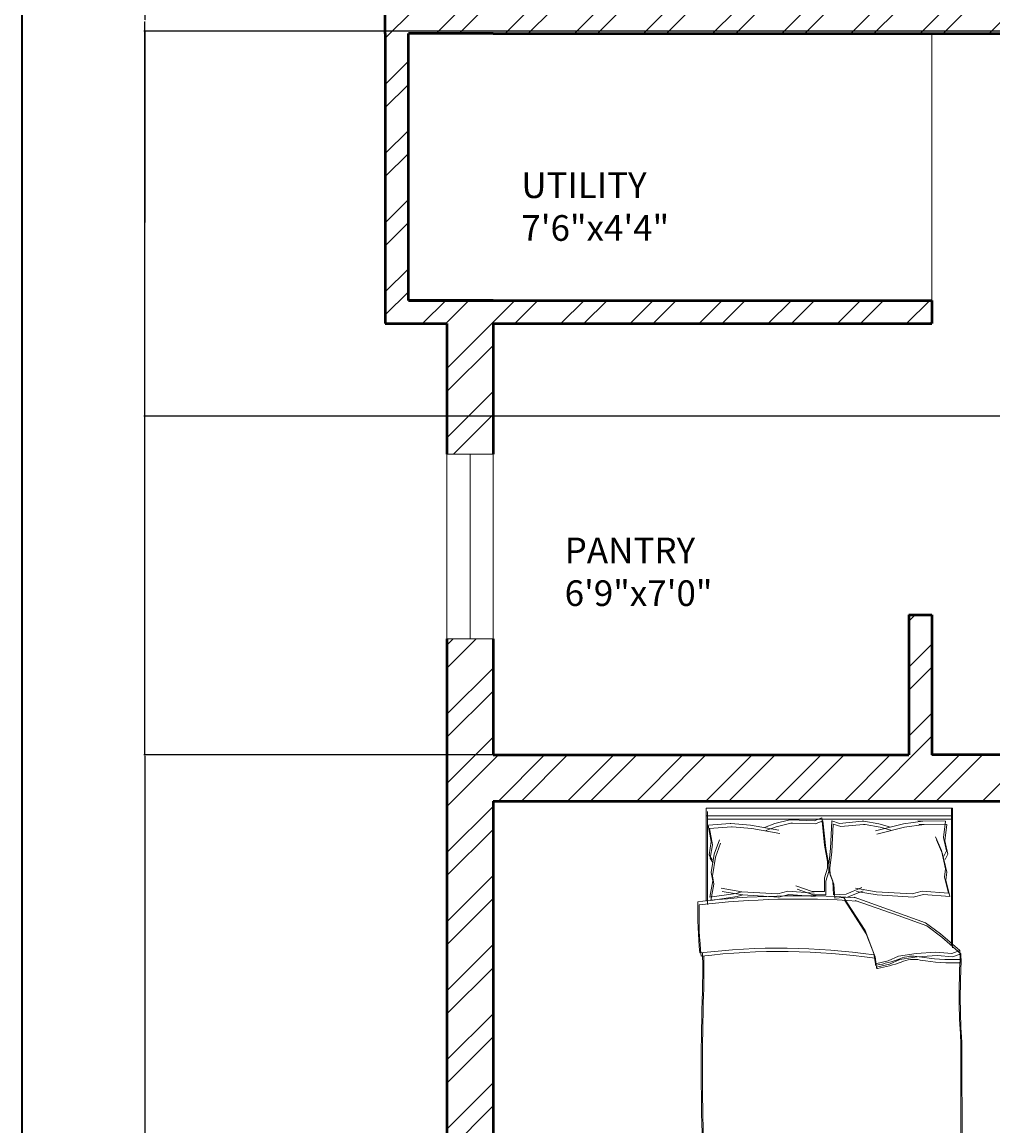
# Model space of a CAD drawing. Units: inches. Extents: x 1896 to 2572, y 1528 to 2474.
# Tile 2 of 10: x 1896 to 2085, y 1818 to 2033. Entities that reach past the tile are written whole.
import ezdxf

# ---------------------------------------------------------------- set-up
doc = ezdxf.new("R2010")
doc.units = ezdxf.units.IN
for name, color, linetype, lineweight in [('A-ANNO-DIMS', 2, 'Continuous', 18), ('A-ANNO-TTLB', 7, 'Continuous', 35), ('A-AREA-IDEN', 7, 'Continuous', 18), ('A-FLOR', 7, 'Continuous', 18), ('A-FURN', 8, 'Continuous', 18), ('A-GLAZ', 131, 'Continuous', 20), ('A-WALL', 7, 'Continuous', 50)]:
    doc.layers.add(name, color=color, linetype=linetype, lineweight=lineweight)
doc.layers.add('A-WALL-PATT', color=215, linetype='Continuous', lineweight=13, true_color=0xa953a0)
doc.styles.get("Standard").update_dxf_attribs({"font": 'arial.ttf'})
doc.dimstyles.get("Standard").update_dxf_attribs({"dimtxt": 0.18, "dimasz": 0.18, "dimexe": 0.18, "dimexo": 0.0625, "dimgap": 0.09, "dimtad": 0, "dimtih": 1, "dimtoh": 1, "dimdec": 4, "dimzin": 0, "dimdsep": 46, "dimtxsty": 'Standard', "dimcen": 0.09, "dimadec": 0, "dimazin": 0, "dimtfac": 1, "dimtdec": 4, "dimtofl": 0, "dimtmove": 0, "dimatfit": 3, "dimfxl": 1, "dimtolj": 1, "dimtzin": 0, "dimarcsym": 0})

# ---------------------------------------------------------------- blocks, each defined once
blk = doc.blocks.new('BED-DOUBLE')
for p, q in [((3.47, 63.33), (3.47, 81.44)), ((3.47, 63.33), (3.47, 81.44)), ((3.47, 81.44), (51.49, 81.44)), ((3.47, 79.91), (51.27, 79.91)), ((3.47, 79.91), (51.26, 79.91)), ((3.7, 62.69), (3.7, 80.8)), ((3.7, 62.69), (3.7, 80.8)), ((24.54, 78.99), (25.98, 79.57)), ((24.54, 78.99), (25.98, 79.57)), ((25.98, 79.57), (26.56, 74.22)), ((25.98, 79.57), (26.56, 74.22)), ((51.26, 81.44), (51.26, 54.83)), ((51.27, 81.44), (51.27, 54.83)), ((51.49, 81.44), (51.49, 80.8)), ((51.49, 80.8), (51.49, 54.19)), ((51.49, 80.8), (51.49, 54.19)), ((3.7, 79.27), (51.49, 79.27)), ((3.7, 79.27), (51.49, 79.27)), ((3.89, 78.13), (4.47, 74.95)), ((3.89, 78.13), (4.47, 74.95)), ((3.9, 78.11), (8.18, 78.43)), ((3.9, 78.11), (8.18, 78.43)), ((4.12, 77.49), (4.7, 74.31)), ((4.12, 77.49), (4.7, 74.31)), ((4.13, 77.47), (8.41, 77.8)), ((4.13, 77.47), (8.41, 77.8)), ((8.18, 78.43), (8.28, 78.42)), ((8.18, 78.43), (8.28, 78.42)), ((8.28, 78.42), (12.11, 78.13)), ((8.28, 78.42), (12.11, 78.13)), ((8.41, 77.8), (8.51, 77.78)), ((8.41, 77.8), (8.51, 77.78)), ((8.51, 77.78), (12.34, 77.49)), ((8.51, 77.78), (12.34, 77.49)), ((12.11, 78.13), (17.6, 77.12)), ((12.11, 78.13), (17.6, 77.12)), ((12.34, 77.49), (17.83, 76.48)), ((12.34, 77.49), (17.83, 76.48)), ((14.85, 77.69), (16.88, 78.42)), ((14.85, 77.69), (16.88, 78.42)), ((15.08, 77.05), (17.11, 77.78)), ((15.08, 77.05), (17.11, 77.78)), ((16.88, 78.42), (19.77, 79.14)), ((16.88, 78.42), (19.77, 79.14)), ((17.11, 77.78), (20, 78.5)), ((17.11, 77.78), (20, 78.5)), ((19.77, 79.14), (20.09, 79.14)), ((19.77, 79.14), (20.09, 79.14)), ((20, 78.5), (20.32, 78.5)), ((20, 78.5), (20.32, 78.5)), ((20.09, 79.14), (24.54, 78.99)), ((20.09, 79.14), (24.54, 78.99)), ((20.32, 78.5), (24.77, 78.36)), ((20.32, 78.5), (24.76, 78.36)), ((24.76, 78.36), (26.21, 78.93)), ((24.77, 78.36), (26.21, 78.93)), ((26.21, 78.93), (26.79, 73.58)), ((26.21, 78.93), (26.79, 73.58)), ((27.98, 78.95), (27.73, 73.58)), ((27.98, 78.95), (27.73, 73.58)), ((28.21, 78.31), (27.96, 72.94)), ((28.2, 78.31), (27.96, 72.94)), ((29.46, 78.46), (27.98, 78.95)), ((29.46, 78.46), (27.98, 78.95)), ((29.68, 77.83), (28.2, 78.31)), ((29.68, 77.83), (28.21, 78.31)), ((33.88, 78.89), (29.46, 78.46)), ((33.88, 78.89), (29.46, 78.46)), ((34.11, 78.25), (29.68, 77.83)), ((34.11, 78.25), (29.68, 77.83)), ((34.2, 78.91), (33.88, 78.89)), ((34.2, 78.91), (33.88, 78.89)), ((34.43, 78.27), (34.11, 78.25)), ((34.43, 78.27), (34.11, 78.25)), ((37.14, 78.37), (34.2, 78.91)), ((37.13, 78.37), (34.2, 78.91)), ((37.36, 77.73), (34.43, 78.27)), ((37.36, 77.73), (34.43, 78.27)), ((41.91, 78.37), (36.49, 77.02)), ((41.91, 78.37), (36.49, 77.02)), ((42.14, 77.73), (36.72, 76.38)), ((42.14, 77.73), (36.72, 76.38)), ((39.2, 77.77), (37.13, 78.37)), ((39.2, 77.77), (37.14, 78.37)), ((39.43, 77.13), (37.36, 77.73)), ((39.43, 77.13), (37.36, 77.73)), ((45.71, 78.9), (41.91, 78.37)), ((45.71, 78.9), (41.91, 78.37)), ((45.94, 78.26), (42.14, 77.73)), ((45.94, 78.26), (42.14, 77.73)), ((50.11, 78.89), (44.71, 78.98)), ((44.71, 78.98), (45.71, 78.9)), ((50.11, 78.89), (44.71, 78.98)), ((44.71, 78.98), (45.71, 78.9)), ((50.34, 78.25), (44.94, 78.34)), ((44.94, 78.34), (45.94, 78.26)), ((50.34, 78.25), (44.94, 78.34)), ((44.94, 78.34), (45.94, 78.26)), ((50.11, 78.89), (49.73, 75.68)), ((50.11, 78.89), (49.73, 75.68)), ((50.34, 78.25), (49.96, 75.04)), ((50.34, 78.25), (49.96, 75.04)), ((49.31, 73.19), (48.13, 75.87)), ((49.31, 73.19), (48.13, 75.87)), ((49.73, 75.68), (50.33, 73.11)), ((49.73, 75.68), (50.33, 73.11)), ((4.47, 74.95), (4.04, 72.34)), ((4.47, 74.95), (4.04, 72.34)), ((4.7, 74.31), (4.27, 71.7)), ((4.7, 74.31), (4.27, 71.7)), ((5.05, 72.49), (6.06, 75.24)), ((5.05, 72.49), (6.06, 75.24)), ((5.28, 71.85), (6.29, 74.6)), ((5.28, 71.85), (6.29, 74.6)), ((26.56, 74.22), (27.14, 71.04)), ((26.56, 74.22), (27.14, 71.04)), ((26.79, 73.58), (27.37, 70.4)), ((26.79, 73.58), (27.37, 70.4)), ((27.73, 73.58), (27.35, 70.37)), ((27.73, 73.58), (27.35, 70.37)), ((49.54, 72.55), (48.36, 75.23)), ((49.54, 72.55), (48.36, 75.23)), ((50.11, 69.61), (49.31, 73.19)), ((50.11, 69.61), (49.31, 73.19)), ((49.96, 75.04), (50.56, 72.47)), ((49.96, 75.04), (50.56, 72.47)), ((4.04, 72.34), (4.62, 71.33)), ((4.04, 72.34), (4.62, 71.33)), ((4.27, 71.7), (4.85, 70.69)), ((4.27, 71.7), (4.85, 70.69)), ((4.47, 68.87), (5.05, 72.49)), ((4.47, 68.87), (5.05, 72.49)), ((4.7, 68.23), (5.28, 71.85)), ((4.7, 68.23), (5.28, 71.85)), ((27.14, 71.04), (27.14, 69.74)), ((27.14, 71.04), (27.14, 69.74)), ((27.96, 72.94), (27.58, 69.73)), ((27.96, 72.94), (27.58, 69.73)), ((50.34, 68.98), (49.54, 72.55)), ((50.34, 68.98), (49.54, 72.55)), ((50.33, 73.11), (49.81, 72.06)), ((50.33, 73.11), (49.81, 72.06)), ((50.56, 72.47), (50.04, 71.42)), ((50.56, 72.47), (50.04, 71.42)), ((4.76, 67.28), (4.47, 68.87)), ((4.76, 67.28), (4.47, 68.87)), ((27.14, 69.74), (26.56, 67.86)), ((27.14, 69.74), (26.56, 67.86)), ((27.37, 69.1), (26.79, 67.22)), ((27.37, 69.1), (26.79, 67.22)), ((27.35, 70.37), (27.44, 69.07)), ((27.35, 70.37), (27.44, 69.07)), ((27.37, 70.4), (27.37, 69.1)), ((27.37, 70.4), (27.37, 69.1)), ((27.44, 69.07), (28.13, 67.23)), ((27.44, 69.07), (28.13, 67.23)), ((27.58, 69.73), (27.66, 68.43)), ((27.58, 69.73), (27.66, 68.43)), ((49.92, 68.01), (50.11, 69.61)), ((49.92, 68.01), (50.11, 69.61)), ((50.15, 67.37), (50.34, 68.98)), ((50.15, 67.37), (50.34, 68.98)), ((4.18, 64.1), (4.76, 67.28)), ((4.18, 64.1), (4.76, 67.28)), ((4.99, 66.64), (4.7, 68.23)), ((4.99, 66.64), (4.7, 68.23)), ((26.56, 67.86), (26.56, 65.18)), ((26.56, 67.86), (26.56, 65.18)), ((26.79, 67.22), (26.79, 64.54)), ((26.79, 67.22), (26.79, 64.54)), ((27.66, 68.43), (28.36, 66.59)), ((27.66, 68.43), (28.36, 66.59)), ((28.13, 67.23), (28.3, 64.55)), ((28.13, 67.23), (28.3, 64.55)), ((50.7, 64.87), (49.92, 68.01)), ((50.7, 64.87), (49.92, 68.01)), ((50.93, 64.23), (50.15, 67.37)), ((50.93, 64.23), (50.15, 67.37)), ((9.28, 64.83), (4.18, 64.1)), ((9.28, 64.83), (4.18, 64.1)), ((4.41, 63.46), (4.99, 66.64)), ((4.41, 63.46), (4.99, 66.64)), ((6.38, 65.81), (10.41, 65.15)), ((6.38, 65.81), (10.41, 65.15)), ((6.61, 65.18), (10.64, 64.51)), ((6.61, 65.18), (10.64, 64.51)), ((10.41, 65.15), (9.28, 64.83)), ((10.41, 65.15), (9.28, 64.83)), ((10.41, 65.15), (17.42, 64.72)), ((10.41, 65.15), (17.42, 64.72)), ((17.42, 64.72), (19.38, 65.27)), ((17.42, 64.72), (19.38, 65.27)), ((17.65, 64.08), (19.61, 64.63)), ((17.65, 64.08), (19.61, 64.63)), ((19.38, 65.27), (24.52, 64.87)), ((19.38, 65.27), (24.52, 64.87)), ((19.61, 64.63), (24.74, 64.23)), ((19.61, 64.63), (24.74, 64.23)), ((24.1, 65.18), (20.96, 66.27)), ((24.1, 65.18), (20.96, 66.27)), ((24.33, 64.54), (21.19, 65.63)), ((24.33, 64.54), (21.19, 65.63)), ((26.56, 65.18), (24.1, 65.18)), ((26.56, 65.18), (24.1, 65.18)), ((26.79, 64.54), (24.33, 64.54)), ((26.79, 64.54), (24.33, 64.54)), ((28.3, 64.55), (30.75, 64.7)), ((28.3, 64.55), (30.75, 64.7)), ((28.36, 66.59), (28.53, 63.91)), ((28.36, 66.59), (28.53, 63.91)), ((30.75, 64.7), (33.82, 65.99)), ((30.75, 64.7), (33.82, 65.99)), ((30.98, 64.06), (34.05, 65.35)), ((30.98, 64.06), (34.05, 65.35)), ((32.56, 65.81), (36.6, 65.15)), ((32.56, 65.81), (36.6, 65.15)), ((32.79, 65.18), (36.82, 64.51)), ((32.79, 65.18), (36.82, 64.51)), ((36.6, 65.15), (43.61, 64.72)), ((36.6, 65.15), (43.61, 64.72)), ((43.61, 64.72), (45.57, 65.27)), ((43.61, 64.72), (45.57, 65.27)), ((43.83, 64.08), (45.79, 64.63)), ((43.83, 64.08), (45.79, 64.63)), ((45.57, 65.27), (50.7, 64.87)), ((45.57, 65.27), (50.7, 64.87)), ((45.79, 64.63), (50.93, 64.23)), ((45.79, 64.63), (50.93, 64.23)), ((9.51, 64.19), (4.41, 63.46)), ((9.51, 64.19), (4.41, 63.46)), ((10.64, 64.51), (9.51, 64.19)), ((10.64, 64.51), (9.51, 64.19)), ((10.64, 64.51), (17.65, 64.08)), ((10.64, 64.51), (17.65, 64.08)), ((28.53, 63.91), (30.98, 64.06)), ((28.53, 63.91), (30.98, 64.06)), ((30.26, 64.06), (34.45, 57.57)), ((30.26, 64.06), (34.45, 57.57)), ((30.49, 63.42), (34.68, 56.93)), ((30.49, 63.42), (34.68, 56.93)), ((40.64, 61.13), (32.31, 64.06)), ((40.64, 61.13), (32.31, 64.06)), ((40.87, 60.49), (32.53, 63.42)), ((40.87, 60.49), (32.53, 63.42)), ((36.82, 64.51), (43.83, 64.08)), ((36.82, 64.51), (43.83, 64.08)), ((46.22, 59.11), (40.64, 61.13)), ((46.22, 59.11), (40.64, 61.13)), ((46.45, 58.48), (40.87, 60.49)), ((46.45, 58.48), (40.87, 60.49)), ((49.16, 56.95), (46.22, 59.11)), ((49.16, 56.95), (46.22, 59.11)), ((49.39, 56.31), (46.45, 58.48)), ((49.39, 56.31), (46.45, 58.48)), ((34.45, 57.57), (36.15, 53.08)), ((34.45, 57.57), (36.15, 53.08)), ((34.68, 56.93), (36.38, 52.44)), ((34.68, 56.93), (36.38, 52.44)), ((52.87, 53.7), (49.16, 56.95)), ((52.87, 53.7), (49.16, 56.95)), ((53.1, 53.06), (49.39, 56.31)), ((53.1, 53.06), (49.39, 56.31)), ((36.15, 53.08), (36.46, 51.07)), ((36.15, 53.08), (36.46, 51.07)), ((36.38, 52.44), (36.69, 50.43)), ((36.38, 52.44), (36.69, 50.43)), ((36.46, 51.07), (38.94, 51.69)), ((36.46, 51.07), (38.94, 51.69)), ((38.94, 51.69), (40.95, 52.61)), ((38.94, 51.69), (40.95, 52.61)), ((39.17, 51.05), (41.18, 51.97)), ((39.17, 51.05), (41.18, 51.97)), ((40.95, 52.61), (44.36, 53.08)), ((40.95, 52.61), (44.36, 53.08)), ((41.18, 51.97), (44.59, 52.44)), ((41.18, 51.97), (44.59, 52.44)), ((44.36, 53.08), (48.23, 53.39)), ((44.36, 53.08), (48.23, 53.39)), ((44.59, 52.44), (48.46, 52.75)), ((44.59, 52.44), (48.46, 52.75)), ((48.23, 53.39), (51.33, 53.08)), ((48.23, 53.39), (51.33, 53.08)), ((48.46, 52.75), (51.56, 52.44)), ((48.46, 52.75), (51.56, 52.44)), ((51.33, 53.08), (52.87, 53.7)), ((51.33, 53.08), (52.87, 53.7)), ((51.56, 52.44), (53.1, 53.06)), ((51.56, 52.44), (53.1, 53.06)), ((52.95, 51.95), (52.87, 53.7, 3.87)), ((52.95, 51.95), (52.87, 53.7, 3.87)), ((53.18, 51.31), (53.1, 53.06, 3.87)), ((53.17, 51.31), (53.1, 53.06, 3.87)), ((36.69, 50.43), (39.17, 51.05)), ((36.69, 50.43), (39.17, 51.05)), ((15.06, 2.2), (39.68, 2.2)), ((15.06, 2.2), (39.68, 2.2)), ((15.29, 1.56), (39.91, 1.56)), ((15.29, 1.56), (39.91, 1.56))]:
    blk.add_line(p, q)
for centre, radius, start, end in [((85.16, 61.35), 83.31, 178.7218, 185.604), ((85.16, 61.35), 83.31, 178.7218, 185.604), ((21.36, -100.61), 164.97, 86.0865, 96.7821), ((21.36, -100.61), 164.97, 86.0865, 96.7821), ((85.39, 60.71), 83.31, 178.7218, 185.604), ((85.39, 60.71), 83.31, 178.7218, 185.604), ((21.59, -101.25), 164.97, 86.0865, 96.7821), ((21.59, -101.25), 164.97, 86.0865, 96.7821), ((17.76, -74.87), 129.02, 81.7845, 96.9006), ((17.76, -74.87), 129.02, 81.7845, 96.9006), ((17.98, -75.51), 129.02, 81.7845, 96.9006), ((17.98, -75.51), 129.02, 81.7845, 96.9006), ((-167.31, 50.27), 170.11, 358.4762, 1.0082), ((-167.31, 50.27), 170.11, 358.4762, 1.0082), ((-167.08, 49.63), 170.11, 358.4762, 1.0082), ((-167.08, 49.63), 170.11, 358.4762, 1.0082), ((31.15, 79.96), 29.65, 280.6617, 289.8806), ((31.15, 79.96), 29.65, 280.6617, 289.8806), ((43.74, 46.38), 6.22, 78.6608, 113.7384), ((43.74, 46.38), 6.22, 78.6608, 113.7384), ((43.97, 45.74), 6.22, 78.6608, 113.7384), ((43.97, 45.74), 6.22, 78.6608, 113.7384), ((51.33, 88.1), 36.18, 259.8763, 272.5657), ((51.33, 88.1), 36.18, 259.8763, 272.5657), ((51.56, 87.46), 36.18, 259.8763, 272.5657), ((51.56, 87.46), 36.18, 259.8763, 272.5657), ((182.27, 45.13), 129.5, 176.9791, 183.8365), ((182.27, 45.13), 129.5, 176.9791, 183.8365), ((36.64, 51), 0.185, 160.2464, 271.1377), ((36.64, 51), 0.185, 160.2464, 271.1377), ((36.86, 50.36), 0.185, 160.2464, 271.1377), ((36.86, 50.36), 0.185, 160.2464, 271.1377), ((31.38, 79.32), 29.65, 280.6617, 289.8806), ((31.38, 79.32), 29.65, 280.6617, 289.8806), ((182.49, 44.49), 129.5, 176.9791, 183.8365), ((182.49, 44.49), 129.5, 176.9791, 183.8365), ((484.82, 30.83), 482.31, 178.2277, 181.7185), ((484.82, 30.83), 482.31, 178.2277, 181.7185), ((485.05, 30.19), 482.31, 178.2277, 181.7185), ((485.05, 30.19), 482.31, 178.2277, 181.7185), ((-4508.74, 13.62), 4561.86, 0.00217, 0.28689), ((-4508.74, 13.62), 4561.86, 0.00217, 0.28689), ((-4508.52, 12.98), 4561.86, 0.00217, 0.28689), ((-4508.52, 12.98), 4561.86, 0.00217, 0.28689), ((-26.9, 16.93), 29.63, 346.0648, 358.9113), ((-26.9, 16.93), 29.63, 346.0648, 358.9113), ((-26.67, 16.29), 29.63, 346.0648, 358.9113), ((-26.67, 16.29), 29.63, 346.0648, 358.9113), ((76.16, 12.78), 23.07, 177.4714, 206.4681), ((76.16, 12.78), 23.07, 177.4714, 206.4681), ((76.39, 12.14), 23.07, 177.4714, 206.4681), ((76.39, 12.14), 23.07, 177.4714, 206.4681), ((-21.66, 11.17), 23.56, 337.9751, 356.652), ((-21.66, 11.17), 23.56, 337.9751, 356.652), ((-21.43, 10.53), 23.56, 337.9751, 356.652), ((-21.43, 10.53), 23.56, 337.9751, 356.652), ((1.09, 1.73), 1.09, 146.1736, 293.4781), ((1.09, 1.73), 1.09, 146.1736, 293.4781), ((21.43, -119.39), 121.76, 92.9958, 99.4091), ((21.43, -119.39), 121.76, 92.9958, 99.4091), ((-17.22, 105.16), 106.46, 283.3832, 287.7053), ((-17.22, 105.16), 106.46, 283.3832, 287.7053), ((-16.99, 104.52), 106.46, 283.3832, 287.7053), ((-16.99, 104.52), 106.46, 283.3832, 287.7053), ((41.15, -130.83), 133.04, 84.4998, 90.6351), ((41.15, -130.83), 133.04, 84.4998, 90.6351), ((54.41, 2.57), 1.1, 242.6588, 356.02), ((54.41, 2.57), 1.1, 242.6588, 356.02), ((1.32, 1.09), 1.09, 146.1736, 293.4781), ((1.32, 1.09), 1.09, 146.1736, 293.4781), ((21.65, -120.03), 121.76, 92.9958, 99.4091), ((21.65, -120.03), 121.76, 92.9958, 99.4091), ((41.38, -131.47), 133.04, 84.4998, 90.6351), ((41.38, -131.47), 133.04, 84.4998, 90.6351), ((54.64, 1.93), 1.1, 242.6588, 356.02), ((54.64, 1.93), 1.1, 242.6588, 356.02)]:
    blk.add_arc(centre, radius, start, end)
blk = doc.blocks.new('*D27')
at = {"layer": 'A-ANNO-DIMS', "color": 0, "lineweight": -2, "transparency": 16777216}
for p, q in [((1987.56, 2175.9), (1919.59, 2175.9)), ((1919.77, 2175.72), (1919.77, 2033.08)), ((1919.77, 1890.08), (1919.77, 2032.72)), ((1987.56, 1889.9), (1919.59, 1889.9))]:
    blk.add_line(p, q, dxfattribs=at)
at = {"layer": 'A-ANNO-DIMS', "color": 0, "transparency": 16777216}
for points in [[(1919.74, 2175.72), (1919.8, 2175.72), (1919.77, 2175.9)], [(1919.74, 1890.08), (1919.8, 1890.08), (1919.77, 1889.9)]]:
    blk.add_solid(points, dxfattribs=at)
at = {"layer": 'Defpoints', "color": 0, "transparency": 16777216}
for p in [(1987.62, 2175.9), (1919.77, 1889.9), (1987.62, 1889.9)]:
    blk.add_point(p, dxfattribs=at)
at = {"layer": 'A-ANNO-DIMS', "color": 0, "transparency": 16777216, "insert": (1919.77, 2032.9), "char_height": 0.18, "attachment_point": 5}
blk.add_mtext('\\A1;286', dxfattribs=at)
blk = doc.blocks.new('*D28')
at = {"layer": 'A-ANNO-DIMS', "color": 0, "lineweight": -2, "transparency": 16777216}
for p, q in [((1987.56, 1889.9), (1919.59, 1889.9)), ((1919.77, 1889.72), (1919.77, 1787.33)), ((1919.77, 1684.58), (1919.77, 1786.97)), ((1978.56, 1684.4), (1919.59, 1684.4))]:
    blk.add_line(p, q, dxfattribs=at)
at = {"layer": 'A-ANNO-DIMS', "color": 0, "transparency": 16777216}
for points in [[(1919.74, 1889.72), (1919.8, 1889.72), (1919.77, 1889.9)], [(1919.74, 1684.58), (1919.8, 1684.58), (1919.77, 1684.4)]]:
    blk.add_solid(points, dxfattribs=at)
at = {"layer": 'Defpoints', "color": 0, "transparency": 16777216}
for p in [(1987.62, 1889.9), (1919.77, 1684.4), (1978.62, 1684.4)]:
    blk.add_point(p, dxfattribs=at)
at = {"layer": 'A-ANNO-DIMS', "color": 0, "transparency": 16777216, "insert": (1919.77, 1787.15), "char_height": 0.18, "attachment_point": 5}
blk.add_mtext('\\A1;205.5', dxfattribs=at)
blk = doc.blocks.new('*D31')
at = {"layer": 'A-ANNO-DIMS', "color": 0, "lineweight": -2, "transparency": 16777216}
for p, q in [((2301.2, 2030.9), (1919.59, 2030.9)), ((1919.77, 2030.72), (1919.77, 1993.58)), ((1919.77, 1956.08), (1919.77, 1993.22)), ((2301.2, 1955.9), (1919.59, 1955.9))]:
    blk.add_line(p, q, dxfattribs=at)
at = {"layer": 'A-ANNO-DIMS', "color": 0, "transparency": 16777216}
for points in [[(1919.74, 2030.72), (1919.8, 2030.72), (1919.77, 2030.9)], [(1919.74, 1956.08), (1919.8, 1956.08), (1919.77, 1955.9)]]:
    blk.add_solid(points, dxfattribs=at)
at = {"layer": 'Defpoints', "color": 0, "transparency": 16777216}
for p in [(1919.77, 2030.9), (2301.26, 2030.9), (2301.26, 1955.9)]:
    blk.add_point(p, dxfattribs=at)
at = {"layer": 'A-ANNO-DIMS', "color": 0, "transparency": 16777216, "insert": (1919.77, 1993.4), "char_height": 0.18, "attachment_point": 5}
blk.add_mtext('\\A1;75', dxfattribs=at)

msp = doc.modelspace()

# ---------------------------------------------------------------- hatches: boundary and pattern name
at = {"layer": 'A-WALL-PATT'}
h = msp.add_hatch(dxfattribs=at)
h.set_pattern_fill('ANSI32', color=256)
h.paths.add_polyline_path([(2071.6224, 2382.3979), (2071.6224, 2422.3979), (2110.6224, 2422.3979), (2110.6224, 2382.3979), (2110.6224, 2357.5961), (2119.6224, 2357.5961), (2119.6224, 2422.3979), (2171.6224, 2422.3979), (2171.6224, 2373.3979), (2193.5093, 2373.3979), (2193.5093, 2377.8979), (2193.5093, 2382.3979), (2180.6224, 2382.3979), (2180.6224, 2431.3979), (2171.6224, 2431.3979), (2119.6224, 2431.3979), (2110.6224, 2431.3979), (2062.6224, 2431.3979), (2062.6224, 2422.3979), (2062.6224, 2382.3979), (1978.6224, 2382.3979), (1978.6224, 2313.0337), (1987.6224, 2313.0337), (1987.6224, 2373.3979), (2062.6224, 2373.3979), (2067.1224, 2373.3979), (2067.1224, 2353.7982), (2071.6224, 2353.8883)])
h.paths.add_polyline_path([(2287.4624, 2382.3979), (2229.5093, 2382.3979), (2229.5093, 2373.3979), (2253.1224, 2373.3979), (2253.1224, 2175.8979), (2247.1039, 2175.8979), (2247.1039, 2166.8979), (2253.1224, 2166.8979), (2253.1224, 2150.8283), (2262.1224, 2150.8283), (2262.1224, 2166.8979), (2262.1224, 2236.8979), (2349.0731, 2236.8979), (2349.0731, 2239.1479), (2349.0731, 2241.3979), (2262.1224, 2241.3979), (2262.1224, 2373.3979), (2287.4624, 2373.3979)])
h.paths.add_polyline_path([(2452.6224, 2382.3979), (2347.4624, 2382.3979), (2347.4624, 2373.3979), (2382.1224, 2373.3979), (2382.1224, 2334.0335), (2386.6224, 2334.0335), (2386.6224, 2373.3979), (2443.6224, 2373.3979), (2443.6224, 2316.2056), (2452.6224, 2316.2056)])
h.paths.add_polyline_path([(2452.6224, 2292.2056), (2448.1224, 2292.2056), (2443.6224, 2292.2056), (2443.6224, 2292.0047), (2443.6224, 2280.9372), (2443.6224, 2268.3979), (2386.6224, 2268.3979), (2386.6224, 2312.4044), (2384.3724, 2312.4044), (2382.1224, 2312.4044), (2382.1224, 2241.3979), (2379.1336, 2241.3979), (2379.1336, 2236.8979), (2386.6224, 2236.8979), (2386.6224, 2263.8979), (2443.6224, 2263.8979), (2443.6224, 2248.8449), (2452.6224, 2248.8449)])
h.paths.add_polyline_path([(2364.1285, 2116.8979), (2262.1224, 2116.8979), (2262.1224, 2120.5401), (2257.6224, 2120.5401), (2253.1224, 2120.5401), (2253.1224, 2107.8979), (2262.1224, 2107.8979), (2269.354, 2107.8979), (2269.354, 2094.0702), (2278.354, 2094.0702), (2278.354, 2107.8979), (2347.6224, 2107.8979), (2347.6224, 2039.8979), (2278.354, 2039.8979), (2278.354, 2054.7605), (2269.354, 2054.7605), (2269.354, 2030.8979), (2278.354, 2030.8979), (2443.6224, 2030.8979), (2443.6224, 2015.198), (2452.6224, 2015.198), (2452.6224, 2030.8979), (2464.6224, 2030.8979), (2469.1224, 2030.8979), (2469.1224, 2117.0352), (2452.6767, 2116.9466), (2452.6285, 2125.8979), (2452.6224, 2125.8979), (2452.6224, 2212.8449), (2443.6224, 2212.8449), (2443.6224, 2116.8979), (2385.832, 2116.8979), (2385.832, 2112.3979), (2385.832, 2107.8979), (2464.6224, 2107.8979), (2464.6224, 2039.8979), (2443.6224, 2039.8979), (2356.6224, 2039.8979), (2356.6224, 2107.8979), (2364.1285, 2107.8979)])
h.paths.add_polyline_path([(2452.6224, 1967.198), (2443.6224, 1967.198), (2443.6224, 1955.8979), (2259.1224, 1955.8979), (2254.6224, 1955.8979), (2254.6224, 1941.6358), (2263.6224, 1941.6358), (2263.6224, 1946.8979), (2379.1224, 1946.8979), (2379.1224, 1913.0204), (2383.6224, 1913.0204), (2383.6224, 1946.8979), (2443.6224, 1946.8979), (2443.6224, 1930.729), (2452.6224, 1930.729)])
h.paths.add_polyline_path([(2469.1224, 1871.8979), (2464.6224, 1871.8979), (2452.6224, 1871.8979), (2452.6224, 1894.729), (2443.6224, 1894.729), (2443.6224, 1871.8979), (2388.1304, 1871.8979), (2388.1304, 1867.3979), (2443.6224, 1867.3979), (2464.6224, 1867.3979), (2464.6224, 1817.8979), (2443.6224, 1817.8979), (2388.1304, 1817.8979), (2388.1304, 1815.6479), (2388.1304, 1813.3979), (2391.1224, 1813.3979), (2391.1224, 1747.8899), (2395.6224, 1747.8899), (2395.6224, 1813.3979), (2443.6224, 1813.3979), (2443.6224, 1781.4434), (2452.6224, 1781.4434), (2452.6224, 1813.3979), (2464.6224, 1813.3979), (2469.1224, 1813.3979)])
h.paths.add_polyline_path([(2263.6224, 1910.9737), (2259.1224, 1910.9737), (2254.6224, 1910.9737), (2254.6224, 1889.8979), (2251.2778, 1889.8979), (2251.2778, 1880.8979), (2254.6224, 1880.8979), (2254.6224, 1817.8979), (2254.6224, 1754.8979), (2254.6224, 1693.3979), (2254.6224, 1684.3979), (2254.6224, 1672.3979), (2200.6224, 1672.3979), (2200.6224, 1684.3979), (2200.6224, 1693.3979), (2200.6224, 1754.8979), (2196.1224, 1754.8979), (2196.1224, 1693.3979), (2150.0488, 1693.3979), (2150.0488, 1684.3979), (2196.1224, 1684.3979), (2196.1224, 1672.3979), (2196.1224, 1667.8979), (2254.6224, 1667.8979), (2259.1224, 1667.8979), (2259.1224, 1693.3979), (2259.1224, 1813.3979), (2353.6224, 1813.3979), (2353.6224, 1815.6479), (2353.6224, 1817.8979), (2263.6224, 1817.8979)])
h.paths.add_polyline_path([(2391.1224, 1693.3979), (2345.6981, 1693.3979), (2345.6981, 1684.3979), (2391.1224, 1684.3979)])
h.paths.add_polyline_path([(2285.6981, 1693.3979), (2259.1224, 1693.3979), (2259.1224, 1684.3979), (2285.6981, 1684.3979), (2285.6981, 1688.8979)], flags=17)
h.paths.add_polyline_path([(2452.6224, 1757.4434), (2448.1224, 1757.4434), (2443.6224, 1757.4434), (2443.6224, 1726.3979), (2395.6224, 1726.3979), (2395.6224, 1728.6572), (2393.3724, 1728.6572), (2391.1224, 1728.6572), (2391.1224, 1717.6723), (2395.6224, 1717.6723), (2395.6224, 1721.8979), (2443.6224, 1721.8979), (2443.6224, 1714.8), (2452.6224, 1714.8)])
h.paths.add_polyline_path([(2452.6224, 1684.3979), (2452.6224, 1690.8), (2443.6224, 1690.8), (2443.6224, 1679.8979), (2443.6224, 1672.3979), (2395.6224, 1672.3979), (2395.6224, 1695.6708), (2391.1224, 1695.5986), (2391.1224, 1672.3979), (2391.1224, 1667.8979), (2452.6224, 1667.8979)])
h.paths.add_polyline_path([(1987.6224, 1880.8979), (2068.6224, 1880.8979), (2125.6224, 1880.8979), (2125.6224, 1788.8466), (2130.1224, 1788.8466), (2130.1224, 1880.8979), (2216.1958, 1880.8979), (2216.1958, 1885.3979), (2216.1958, 1889.8979), (2208.1224, 1889.8979), (2208.1224, 1996.3717), (2203.6224, 1996.3717), (2199.1224, 1996.3717), (2199.1224, 1889.8979), (2073.1224, 1889.8979), (2073.1224, 1917.1874), (2068.6224, 1917.1874), (2068.6224, 1889.8979), (1987.6224, 1889.8979), (1987.6224, 1912.4976), (1978.6224, 1912.4976), (1978.6224, 1805.5193), (1987.6224, 1805.5193)])
h.paths.add_polyline_path([(2019.9303, 1754.8979), (1987.6224, 1754.8979), (1966.6224, 1754.8979), (1966.6224, 1801.0193), (1987.6224, 1801.0193), (1987.6224, 1805.5193), (1962.1224, 1805.5193), (1962.1224, 1750.3979), (1966.6224, 1750.3979), (1978.6224, 1750.3979), (1987.6224, 1750.3979), (2019.9303, 1750.3979)])
h.paths.add_polyline_path([(2135.5566, 1754.8979), (2130.1224, 1754.8979), (2130.1224, 1758.052), (2127.8724, 1758.052), (2125.6224, 1758.052), (2125.6224, 1754.8979), (2068.6224, 1754.8979), (2043.2292, 1754.8979), (2043.2292, 1750.3979), (2068.6224, 1750.3979), (2098.6224, 1750.3979), (2098.6224, 1693.3979), (2068.6224, 1693.3979), (1987.6224, 1693.3979), (1987.6224, 1707.3003), (1983.1224, 1707.3003), (1978.6224, 1707.3003), (1978.6224, 1684.3979), (2068.6224, 1684.3979), (2126.0488, 1684.3979), (2126.0488, 1688.8979), (2126.0488, 1693.3979), (2103.1224, 1693.3979), (2103.1224, 1750.3979), (2130.1224, 1750.3979), (2135.5566, 1750.3979)])
h.paths.add_polyline_path([(1987.6224, 1750.3979), (1978.6224, 1750.3979), (1978.6224, 1731.3003), (1987.6224, 1731.3003)], flags=0)
h.paths.add_polyline_path([(1987.6224, 1973.8979), (2068.6224, 1973.8979), (2073.1224, 1973.8979), (2073.1224, 1978.3979), (1971.1224, 1978.3979), (1971.1224, 2030.3979), (1978.6224, 2030.3979), (1987.6224, 2030.3979), (2104.9199, 2030.3979), (2104.9199, 2032.6479), (2104.9199, 2034.8979), (1987.6224, 2034.8979), (1971.1224, 2034.8979), (1971.1224, 2085.8979), (2003.6464, 2085.8979), (2003.6464, 2090.3979), (1987.6224, 2090.3979), (1987.6224, 2166.8979), (2115.1224, 2166.8979), (2137.6224, 2166.8979), (2137.6224, 2114.4229), (2142.1224, 2114.4229), (2142.1224, 2124.8979), (2153.5306, 2124.8979), (2153.5306, 2127.1479), (2153.5306, 2129.3979), (2142.1224, 2129.3979), (2142.1224, 2166.8979), (2199.1224, 2166.8979), (2199.1224, 2129.3979), (2177.5306, 2129.3979), (2177.5306, 2124.8979), (2199.1224, 2124.8979), (2199.1224, 2034.8979), (2142.1224, 2034.8979), (2142.1224, 2091.6671), (2139.8724, 2091.6671), (2137.6224, 2091.6671), (2137.6224, 2034.8979), (2133.8326, 2034.8979), (2133.8326, 2030.3979), (2137.6224, 2030.3979), (2142.1224, 2030.3979), (2199.1224, 2030.3979), (2199.1224, 2024.2654), (2208.1224, 2024.2654), (2208.1224, 2030.3979), (2208.1224, 2166.8979), (2214.5775, 2166.8979), (2214.5775, 2171.3979), (2214.5775, 2175.8979), (2115.1224, 2175.8979), (2115.1224, 2329.9154), (2112.4137, 2329.9154), (2110.6224, 2329.9154), (2110.6224, 2175.8979), (2082.1224, 2175.8979), (2082.1224, 2202.6443), (2079.8724, 2202.6443), (2077.6224, 2202.6443), (2077.6224, 2175.8979), (1987.6224, 2175.8979), (1987.6224, 2191.3531), (1983.1224, 2191.3531), (1978.6224, 2191.3531), (1978.6224, 2090.3979), (1966.6224, 2090.3979), (1966.6224, 2085.8979), (1966.6224, 2030.3979), (1966.6224, 1973.8979), (1978.6224, 1973.8979), (1978.6224, 1948.4976), (1983.1224, 1948.4976), (1987.6224, 1948.4976)])
h.paths.add_polyline_path([(1987.6224, 2253.0337), (1983.1224, 2253.0337), (1978.6224, 2253.0337), (1978.6224, 2215.3531), (1987.6224, 2215.3531), (1987.6224, 2224.8979), (2077.6224, 2224.8979), (2077.6224, 2221.9854), (2082.1224, 2221.9854), (2082.1224, 2229.3979), (1987.6224, 2229.3979)], flags=17)
h.paths.add_polyline_path([(2220.5047, 1978.7278), (2253.7278, 1978.7278), (2253.7278, 1997.3851), (2220.5047, 1997.3851)], flags=9)
h.paths.add_polyline_path([(2303.6746, 2064.9806), (2320.5334, 2064.9806), (2320.5334, 2075.2842), (2303.6746, 2075.2842)], flags=25)

# ---------------------------------------------------------------- linework, layer by layer
at = {"layer": 'A-ANNO-TTLB'}
msp.add_lwpolyline([(1895.84, 2455.9668), (2571.702, 2455.9668), (2571.702, 1527.8833), (1895.84, 1527.8833)], close=True, dxfattribs=at)
at = {"layer": 'A-FLOR'}
msp.add_line((2073.1224, 1978.3979), (2073.1224, 2030.3979), dxfattribs=at)
at = {"layer": 'A-GLAZ'}
for p, q in [((1987.6224, 1948.4976), (1978.6224, 1948.4976)), ((1978.6224, 1948.4976), (1983.1224, 1948.4976)), ((1978.6224, 1948.4976), (1978.6224, 1912.4976)), ((1983.1224, 1948.4976), (1983.1224, 1912.4976)), ((1987.6224, 1948.4976), (1987.6224, 1912.4976)), ((1983.1224, 1912.4976), (1978.6224, 1912.4976)), ((1978.6224, 1912.4976), (1987.6224, 1912.4976))]:
    msp.add_line(p, q, dxfattribs=at)
at = {"layer": 'A-WALL'}
for p, q in [((1966.6224, 2030.3979), (1966.6224, 2085.8979)), ((1966.6224, 2030.3979), (1966.6224, 1973.8979)), ((1978.6224, 2030.3979), (1971.1224, 2030.3979)), ((1971.1224, 1978.3979), (1971.1224, 2030.3979)), ((1987.6224, 2030.3979), (1978.6224, 2030.3979)), ((1987.6224, 2030.3979), (2104.9199, 2030.3979)), ((1971.1224, 1978.3979), (2073.1224, 1978.3979)), ((1987.6224, 1978.3979), (1971.1224, 1978.3979)), ((2073.1224, 1978.3979), (2073.1224, 1973.8979)), ((1966.6224, 1973.8979), (1978.6224, 1973.8979)), ((1978.6224, 1973.8979), (1978.6224, 1948.4976)), ((1987.6224, 1973.8979), (2068.6224, 1973.8979)), ((1987.6224, 1973.8979), (1987.6224, 1948.4976)), ((2068.6224, 1973.8979), (2073.1224, 1973.8979)), ((2068.6224, 1917.1874), (2068.6224, 1889.8979)), ((2068.6224, 1917.1874), (2073.1224, 1917.1874)), ((2073.1224, 1917.1874), (2073.1224, 1889.8979)), ((1978.6224, 1912.4976), (1978.6224, 1805.5193)), ((1987.6224, 1912.4976), (1987.6224, 1889.8979)), ((1987.6224, 1889.8979), (2068.6224, 1889.8979)), ((2199.1224, 1889.8979), (2073.1224, 1889.8979)), ((1987.6224, 1880.8979), (2068.6224, 1880.8979)), ((1987.6224, 1880.8979), (1987.6224, 1754.8979)), ((2068.6224, 1880.8979), (2125.6224, 1880.8979))]:
    msp.add_line(p, q, dxfattribs=at)

# ---------------------------------------------------------------- block references
at = {"layer": 'A-FURN'}
msp.add_blockref('BED-DOUBLE', (2025.6685, 1798.0776), dxfattribs=at)

# ---------------------------------------------------------------- texts
at = {"layer": 'A-AREA-IDEN', "char_height": 5, "attachment_point": 1}
for s, width, insert in [('UTILITY\\P7\'6"x4\'4"', 104.002054, (1993.1284, 2003.3674)), ('PANTRY\\P6\'9"x7\'0"', 128.101663, (2001.5668, 1932.2236))]:
    msp.add_mtext_dynamic_manual_height_columns(s, width=width, gutter_width=12.5, heights=[0], dxfattribs=dict(at, insert=insert))

# ---------------------------------------------------------------- dimensions: what is measured, and where the dimension line sits
at = {"layer": 'A-ANNO-DIMS'}
for base, p1, p2, override, picture, middle in [((1919.7724, 1889.8979), (1987.6224, 2175.8979), (1987.6224, 1889.8979), {"dimdec": 0, "dimlfac": 1, "dimrnd": 0, "dimzin": 0, "dimdsep": 46, "dimlunit": 2}, '*D27', (1919.7724, 2032.8979)), ((1919.7724, 2030.8979), (2301.2636, 1955.8979), (2301.2636, 2030.8979), {"dimdec": 0, "dimlfac": 1, "dimrnd": 0, "dimzin": 0, "dimdsep": 46, "dimlunit": 2}, '*D31', (1919.7724, 1993.3979)), ((1919.7724, 1684.3979), (1987.6224, 1889.8979), (1978.6224, 1684.3979), {"dimdec": 1, "dimlfac": 1, "dimrnd": 0, "dimzin": 0, "dimdsep": 46, "dimlunit": 2}, '*D28', (1919.7724, 1787.1479))]:
    dim = msp.add_linear_dim(base=base, p1=p1, p2=p2, angle=90, dimstyle='Standard', override=override, dxfattribs=at)
    dim.commit()
    dim.dimension.update_dxf_attribs({"geometry": picture, "text_midpoint": middle})

doc.saveas('drawing.dxf')
